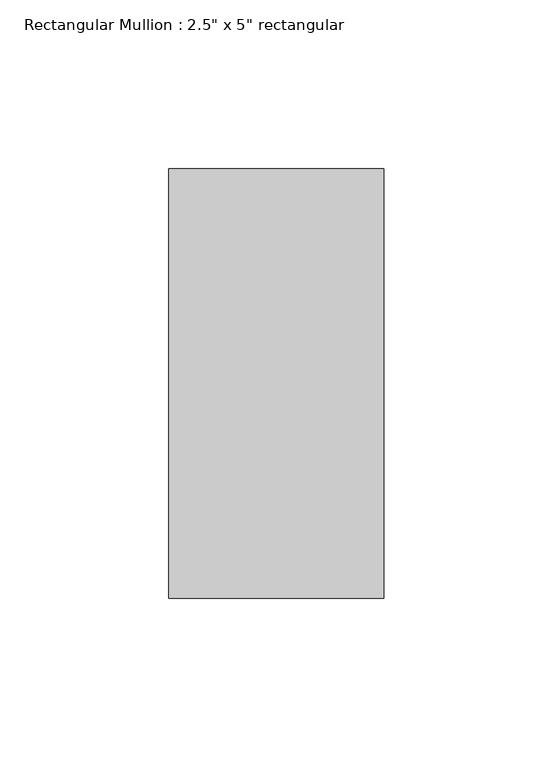
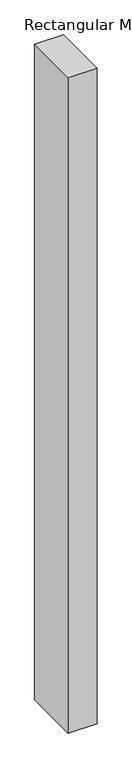
"""IFC4 building model written with IfcOpenShell, lengths in millimetres: member geometry."""

from ifc_helpers import new_model, si_unit, frame, origin, place, context, project, spatial, polyline, outline, extrude, source, transform, mapped, element, save


def member_b4577db3(model_context):
    return source(origin(), model_context, "Body", "SweptSolid", [
        extrude(outline(polyline([(0.0, 63.5), (0.0, -63.5), (-63.5, -63.5), (-63.5, 63.5), (0.0, 63.5)])), frame((0.0, 0.0, -1521.1896321), z_axis=(0.0, 0.0, 1.0), x_axis=(1.0, 0.0, 0.0)), (0.0, 0.0, 1.0), 1521.1896321),
    ])


if __name__ == "__main__":
    model = new_model("IFC4")
    model_context = context("Model", 3, world=origin())
    ifc_project = project(units=[si_unit("LENGTHUNIT", "METRE", prefix="MILLI")], contexts=[model_context])
    site = spatial("IfcSite", under=ifc_project)
    building = spatial("IfcBuilding", under=site)
    placement = place(None, origin())
    member_shape = member_b4577db3(model_context)
    element("IfcMember", 1, ObjectType="Rectangular Mullion : 2.5\" x 5\" rectangular", at=placement, inside=building, context=model_context, shape_type="MappedRepresentation", body=[
        mapped(member_shape, transform((0.0, 0.0, 0.0), x_axis=(1.0, 0.0, 0.0), y_axis=(0.0, 1.0, 0.0), z_axis=(0.0, 0.0, 1.0))),
    ])
    save(model, "model.ifc")

# Revit data of these elements
# Type "Rectangular Mullion : 2.5\" x 5\" rectangular"
#   built-in parameter 1007304 = 0.416667 (stored number, unit not read)
#   built-in parameter 1007301 = 0.104167 (stored number, unit not read)
#   built-in parameter 1007300 = 0.104167 (stored number, unit not read)
# Element 1 (IfcMember, "Rectangular Mullion : 2.5\" x 5\" rectangular")
#   Materials on its faces: "Aluminum"
# Materials
#   "Aluminum": class "Metal", colour RGB 247 247 247, transparency 0, Description = "Aluminum 6061", Cost = 0
